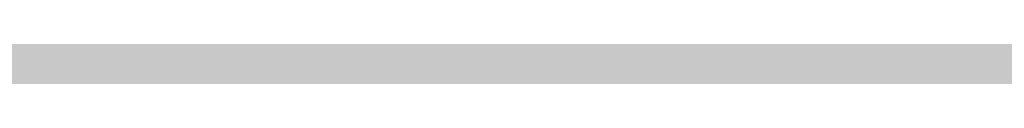
# Model space of a CAD drawing. Units: millimetres. Extents: x -22994 to 29398, y -19990 to 20176.
# Tile 89 of 135: x 229.428 to 230.597, y 83.505 to 83.535. Entities that reach past the tile are written whole.
import ezdxf
from ezdxf import colors
from ezdxf.entities.mleader import LeaderData, LeaderLine
from ezdxf.math import Vec2, Vec3

# ---------------------------------------------------------------- set-up
doc = ezdxf.new("R2010")
doc.units = ezdxf.units.MM
doc.header["$MEASUREMENT"] = 0
doc.layers.add('M-ANNO-TEXT', color=7, linetype='Continuous', lineweight=25)
doc.layers.add('M-DIMS', color=2, linetype='Continuous', lineweight=18)
doc.styles.get("Standard").update_dxf_attribs({"font": 'arial.ttf'})
doc.dimstyles.get("Standard").update_dxf_attribs({"dimtxt": 0.18, "dimasz": 10000, "dimexe": 0.18, "dimexo": 0.0625, "dimgap": 0.09, "dimtad": 0, "dimtih": 1, "dimtoh": 1, "dimdec": 0, "dimzin": 0, "dimdsep": 46, "dimtxsty": 'Standard', "dimcen": 0.09, "dimadec": 0, "dimazin": 0, "dimtfac": 1, "dimtdec": 0, "dimtofl": 0, "dimtmove": 0, "dimatfit": 3, "dimfxl": 1, "dimtolj": 1, "dimtzin": 0, "dimlwd": 30, "dimarcsym": 0})

# ---------------------------------------------------------------- blocks, each defined once
blk = doc.blocks.new('*D2')
at = {"layer": 'Defpoints', "color": 0, "transparency": 16777216}
for p in [(6.6773, 10.2713), (290.852, 10.2713), (290.852, -5.0787)]:
    blk.add_point(p, dxfattribs=at)
at = {"layer": 'M-DIMS', "color": 0, "lineweight": -2, "transparency": 16777216}
for p, q in [((6.6773, 10.2088), (6.6773, -5.2587)), ((290.852, 10.2088), (290.852, -5.2587))]:
    blk.add_line(p, q, dxfattribs=at)
at = {"layer": 'M-DIMS', "color": 0, "lineweight": 30, "transparency": 16777216}
for p, q in [((-9993.3227, -5.0787), (-19993.3227, -5.0787)), ((10290.852, -5.0787), (20290.852, -5.0787))]:
    blk.add_line(p, q, dxfattribs=at)
at = {"layer": 'M-DIMS', "color": 0, "transparency": 16777216}
for points in [[(-9993.3227, 1661.5879), (-9993.3227, -1671.7454), (6.6773, -5.0787)], [(10290.852, 1661.5879), (10290.852, -1671.7454), (290.852, -5.0787)]]:
    blk.add_solid(points, dxfattribs=at)
at = {"layer": 'M-DIMS', "color": 0, "transparency": 16777216, "insert": (148.7647, -5.0787), "char_height": 0.18, "attachment_point": 5}
blk.add_mtext('\\A1;284.2', dxfattribs=at)
blk = doc.blocks.new('*D3')
at = {"layer": 'Defpoints', "color": 0, "transparency": 16777216}
for p in [(110.2647, 204.1654), (110.2647, 176.3662), (95.8327, 127.967)]:
    blk.add_point(p, dxfattribs=at)
at = {"layer": 'M-DIMS', "color": 0, "lineweight": -2, "transparency": 16777216}
for p, q in [((95.8327, 128.0295), (95.8327, 204.3454)), ((110.2647, 176.4287), (110.2647, 204.3454))]:
    blk.add_line(p, q, dxfattribs=at)
at = {"layer": 'M-DIMS', "color": 0, "lineweight": 30, "transparency": 16777216}
for p, q in [((-9904.1673, 204.1654), (-19904.1673, 204.1654)), ((10110.2647, 204.1654), (20110.2647, 204.1654))]:
    blk.add_line(p, q, dxfattribs=at)
at = {"layer": 'M-DIMS', "color": 0, "transparency": 16777216}
for points in [[(-9904.1673, 1870.8321), (-9904.1673, -1462.5013), (95.8327, 204.1654)], [(10110.2647, 1870.8321), (10110.2647, -1462.5013), (110.2647, 204.1654)]]:
    blk.add_solid(points, dxfattribs=at)
at = {"layer": 'M-DIMS', "color": 0, "transparency": 16777216, "insert": (103.0487, 204.1654), "char_height": 0.18, "attachment_point": 5}
blk.add_mtext('\\A1;14.432', dxfattribs=at)
blk = doc.blocks.new('*D4')
at = {"layer": 'Defpoints', "color": 0, "transparency": 16777216}
for p in [(116.2647, 204.1654), (110.2647, 176.3662), (116.2647, 176.3662)]:
    blk.add_point(p, dxfattribs=at)
at = {"layer": 'M-DIMS', "color": 0, "lineweight": -2, "transparency": 16777216}
for p, q in [((110.2647, 176.4287), (110.2647, 204.3454)), ((116.2647, 176.4287), (116.2647, 204.3454))]:
    blk.add_line(p, q, dxfattribs=at)
at = {"layer": 'M-DIMS', "color": 0, "lineweight": 30, "transparency": 16777216}
for p, q in [((-9889.7353, 204.1654), (-19889.7353, 204.1654)), ((10116.2647, 204.1654), (20116.2647, 204.1654))]:
    blk.add_line(p, q, dxfattribs=at)
at = {"layer": 'M-DIMS', "color": 0, "transparency": 16777216}
for points in [[(-9889.7353, 1870.8321), (-9889.7353, -1462.5013), (110.2647, 204.1654)], [(10116.2647, 1870.8321), (10116.2647, -1462.5013), (116.2647, 204.1654)]]:
    blk.add_solid(points, dxfattribs=at)
at = {"layer": 'M-DIMS', "color": 0, "transparency": 16777216, "insert": (113.2647, 204.1654), "char_height": 0.18, "attachment_point": 5}
blk.add_mtext('\\A1;6', dxfattribs=at)
blk = doc.blocks.new('*D5')
at = {"layer": 'Defpoints', "color": 0, "transparency": 16777216}
for p in [(181.2647, 204.1654), (116.2647, 176.3662), (181.2647, 176.3662)]:
    blk.add_point(p, dxfattribs=at)
at = {"layer": 'M-DIMS', "color": 0, "lineweight": -2, "transparency": 16777216}
for p, q in [((116.2647, 176.4287), (116.2647, 204.3454)), ((181.2647, 176.4287), (181.2647, 204.3454))]:
    blk.add_line(p, q, dxfattribs=at)
at = {"layer": 'M-DIMS', "color": 0, "lineweight": 30, "transparency": 16777216}
for p, q in [((-9883.7353, 204.1654), (-19883.7353, 204.1654)), ((10181.2647, 204.1654), (20181.2647, 204.1654))]:
    blk.add_line(p, q, dxfattribs=at)
at = {"layer": 'M-DIMS', "color": 0, "transparency": 16777216}
for points in [[(-9883.7353, 1870.8321), (-9883.7353, -1462.5013), (116.2647, 204.1654)], [(10181.2647, 1870.8321), (10181.2647, -1462.5013), (181.2647, 204.1654)]]:
    blk.add_solid(points, dxfattribs=at)
at = {"layer": 'M-DIMS', "color": 0, "transparency": 16777216, "insert": (148.7647, 204.1654), "char_height": 0.18, "attachment_point": 5}
blk.add_mtext('\\A1;65', dxfattribs=at)
blk = doc.blocks.new('*D6')
at = {"layer": 'Defpoints', "color": 0, "transparency": 16777216}
for p in [(187.2647, 204.1654), (181.2647, 176.3662), (187.2647, 176.3662)]:
    blk.add_point(p, dxfattribs=at)
at = {"layer": 'M-DIMS', "color": 0, "lineweight": -2, "transparency": 16777216}
for p, q in [((181.2647, 176.4287), (181.2647, 204.3454)), ((187.2647, 176.4287), (187.2647, 204.3454))]:
    blk.add_line(p, q, dxfattribs=at)
at = {"layer": 'M-DIMS', "color": 0, "lineweight": 30, "transparency": 16777216}
for p, q in [((-9818.7353, 204.1654), (-19818.7353, 204.1654)), ((10187.2647, 204.1654), (20187.2647, 204.1654))]:
    blk.add_line(p, q, dxfattribs=at)
at = {"layer": 'M-DIMS', "color": 0, "transparency": 16777216}
for points in [[(-9818.7353, 1870.8321), (-9818.7353, -1462.5013), (181.2647, 204.1654)], [(10187.2647, 1870.8321), (10187.2647, -1462.5013), (187.2647, 204.1654)]]:
    blk.add_solid(points, dxfattribs=at)
at = {"layer": 'M-DIMS', "color": 0, "transparency": 16777216, "insert": (184.2647, 204.1654), "char_height": 0.18, "attachment_point": 5}
blk.add_mtext('\\A1;6', dxfattribs=at)
blk = doc.blocks.new('*D7')
at = {"layer": 'Defpoints', "color": 0, "transparency": 16777216}
for p in [(201.6967, 204.1654), (187.2647, 176.3662), (201.6967, 127.967)]:
    blk.add_point(p, dxfattribs=at)
at = {"layer": 'M-DIMS', "color": 0, "lineweight": -2, "transparency": 16777216}
for p, q in [((187.2647, 176.4287), (187.2647, 204.3454)), ((201.6967, 128.0295), (201.6967, 204.3454))]:
    blk.add_line(p, q, dxfattribs=at)
at = {"layer": 'M-DIMS', "color": 0, "lineweight": 30, "transparency": 16777216}
for p, q in [((-9812.7353, 204.1654), (-19812.7353, 204.1654)), ((10201.6967, 204.1654), (20201.6967, 204.1654))]:
    blk.add_line(p, q, dxfattribs=at)
at = {"layer": 'M-DIMS', "color": 0, "transparency": 16777216}
for points in [[(-9812.7353, 1870.8321), (-9812.7353, -1462.5013), (187.2647, 204.1654)], [(10201.6967, 1870.8321), (10201.6967, -1462.5013), (201.6967, 204.1654)]]:
    blk.add_solid(points, dxfattribs=at)
at = {"layer": 'M-DIMS', "color": 0, "transparency": 16777216, "insert": (194.4807, 204.1654), "char_height": 0.18, "attachment_point": 5}
blk.add_mtext('\\A1;14.432', dxfattribs=at)
blk = doc.blocks.new('*D8')
at = {"layer": 'Defpoints', "color": 0, "transparency": 16777216}
for p in [(227.6485, 204.1654), (227.6485, 146.7296), (201.6967, 127.967)]:
    blk.add_point(p, dxfattribs=at)
at = {"layer": 'M-DIMS', "color": 0, "lineweight": -2, "transparency": 16777216}
for p, q in [((201.6967, 128.0295), (201.6967, 204.3454)), ((227.6485, 146.7921), (227.6485, 204.3454))]:
    blk.add_line(p, q, dxfattribs=at)
at = {"layer": 'M-DIMS', "color": 0, "lineweight": 30, "transparency": 16777216}
for p, q in [((-9798.3033, 204.1654), (-19798.3033, 204.1654)), ((10227.6485, 204.1654), (20227.6485, 204.1654))]:
    blk.add_line(p, q, dxfattribs=at)
at = {"layer": 'M-DIMS', "color": 0, "transparency": 16777216}
for points in [[(-9798.3033, 1870.8321), (-9798.3033, -1462.5013), (201.6967, 204.1654)], [(10227.6485, 1870.8321), (10227.6485, -1462.5013), (227.6485, 204.1654)]]:
    blk.add_solid(points, dxfattribs=at)
at = {"layer": 'M-DIMS', "color": 0, "transparency": 16777216, "insert": (214.6726, 204.1654), "char_height": 0.18, "attachment_point": 5}
blk.add_mtext('\\A1;25.95', dxfattribs=at)
blk = doc.blocks.new('*D9')
at = {"layer": 'Defpoints', "color": 0, "transparency": 16777216}
for p in [(187.2647, 176.3662), (306.202, 176.3662), (290.852, 10.2713)]:
    blk.add_point(p, dxfattribs=at)
at = {"layer": 'M-DIMS', "color": 0, "lineweight": 30, "transparency": 16777216}
for p, q in [((306.202, 10176.3662), (306.202, 20176.3662)), ((306.202, -9989.7287), (306.202, -19989.7287))]:
    blk.add_line(p, q, dxfattribs=at)
at = {"layer": 'M-DIMS', "color": 0, "lineweight": -2, "transparency": 16777216}
for p, q in [((187.3272, 176.3662), (306.382, 176.3662)), ((290.9145, 10.2713), (306.382, 10.2713))]:
    blk.add_line(p, q, dxfattribs=at)
at = {"layer": 'M-DIMS', "color": 0, "transparency": 16777216}
for points in [[(-1360.4646, 10176.3662), (1972.8687, 10176.3662), (306.202, 176.3662)], [(-1360.4646, -9989.7287), (1972.8687, -9989.7287), (306.202, 10.2713)]]:
    blk.add_solid(points, dxfattribs=at)
at = {"layer": 'M-DIMS', "color": 0, "transparency": 16777216, "insert": (306.202, 93.3187), "char_height": 0.18, "attachment_point": 5}
blk.add_mtext('\\A1;166.1', dxfattribs=at)
blk = doc.blocks.new('*D10')
at = {"layer": 'Defpoints', "color": 0, "transparency": 16777216}
for p in [(125.6498, 136.0713), (133.3459, 136.0713), (133.3459, -5.0787)]:
    blk.add_point(p, dxfattribs=at)
at = {"layer": 'M-DIMS', "color": 0, "lineweight": -2, "transparency": 16777216}
for p, q in [((125.6498, 136.0088), (125.6498, -5.2587)), ((133.3459, 136.0088), (133.3459, -5.2587))]:
    blk.add_line(p, q, dxfattribs=at)
at = {"layer": 'M-DIMS', "color": 0, "lineweight": 30, "transparency": 16777216}
for p, q in [((-9874.3502, -5.0787), (-19874.3502, -5.0787)), ((10133.3459, -5.0787), (20133.3459, -5.0787))]:
    blk.add_line(p, q, dxfattribs=at)
at = {"layer": 'M-DIMS', "color": 0, "transparency": 16777216}
for points in [[(-9874.3502, 1661.5879), (-9874.3502, -1671.7454), (125.6498, -5.0787)], [(10133.3459, 1661.5879), (10133.3459, -1671.7454), (133.3459, -5.0787)]]:
    blk.add_solid(points, dxfattribs=at)
at = {"layer": 'M-DIMS', "color": 0, "transparency": 16777216, "insert": (129.4978, -5.0787), "char_height": 0.18, "attachment_point": 5}
blk.add_mtext('\\A1;7.696', dxfattribs=at)
blk = doc.blocks.new('*D11')
at = {"layer": 'Defpoints', "color": 0, "transparency": 16777216}
for p in [(133.3459, 136.0713), (135.6498, 136.0713), (135.6498, -5.0787)]:
    blk.add_point(p, dxfattribs=at)
at = {"layer": 'M-DIMS', "color": 0, "lineweight": -2, "transparency": 16777216}
for p, q in [((133.3459, 136.0088), (133.3459, -5.2587)), ((135.6498, 136.0088), (135.6498, -5.2587))]:
    blk.add_line(p, q, dxfattribs=at)
at = {"layer": 'M-DIMS', "color": 0, "lineweight": 30, "transparency": 16777216}
for p, q in [((-9866.6541, -5.0787), (-19866.6541, -5.0787)), ((10135.6498, -5.0787), (20135.6498, -5.0787))]:
    blk.add_line(p, q, dxfattribs=at)
at = {"layer": 'M-DIMS', "color": 0, "transparency": 16777216}
for points in [[(-9866.6541, 1661.5879), (-9866.6541, -1671.7454), (133.3459, -5.0787)], [(10135.6498, 1661.5879), (10135.6498, -1671.7454), (135.6498, -5.0787)]]:
    blk.add_solid(points, dxfattribs=at)
at = {"layer": 'M-DIMS', "color": 0, "transparency": 16777216, "insert": (134.4978, -5.0787), "char_height": 0.18, "attachment_point": 5}
blk.add_mtext('\\A1;2.304', dxfattribs=at)
blk = doc.blocks.new('*D12')
at = {"layer": 'Defpoints', "color": 0, "transparency": 16777216}
for p in [(135.6498, 136.0713), (145.6498, 136.0713), (145.6498, -5.0787)]:
    blk.add_point(p, dxfattribs=at)
at = {"layer": 'M-DIMS', "color": 0, "lineweight": -2, "transparency": 16777216}
for p, q in [((135.6498, 136.0088), (135.6498, -5.2587)), ((145.6498, 136.0088), (145.6498, -5.2587))]:
    blk.add_line(p, q, dxfattribs=at)
at = {"layer": 'M-DIMS', "color": 0, "lineweight": 30, "transparency": 16777216}
for p, q in [((-9864.3502, -5.0787), (-19864.3502, -5.0787)), ((10145.6498, -5.0787), (20145.6498, -5.0787))]:
    blk.add_line(p, q, dxfattribs=at)
at = {"layer": 'M-DIMS', "color": 0, "transparency": 16777216}
for points in [[(-9864.3502, 1661.5879), (-9864.3502, -1671.7454), (135.6498, -5.0787)], [(10145.6498, 1661.5879), (10145.6498, -1671.7454), (145.6498, -5.0787)]]:
    blk.add_solid(points, dxfattribs=at)
at = {"layer": 'M-DIMS', "color": 0, "transparency": 16777216, "insert": (140.6498, -5.0787), "char_height": 0.18, "attachment_point": 5}
blk.add_mtext('\\A1;10', dxfattribs=at)
blk = doc.blocks.new('*D13')
at = {"layer": 'Defpoints', "color": 0, "transparency": 16777216}
for p in [(145.6498, 136.0713), (155.6498, 136.0713), (155.6498, -5.0787)]:
    blk.add_point(p, dxfattribs=at)
at = {"layer": 'M-DIMS', "color": 0, "lineweight": -2, "transparency": 16777216}
for p, q in [((145.6498, 136.0088), (145.6498, -5.2587)), ((155.6498, 136.0088), (155.6498, -5.2587))]:
    blk.add_line(p, q, dxfattribs=at)
at = {"layer": 'M-DIMS', "color": 0, "lineweight": 30, "transparency": 16777216}
for p, q in [((-9854.3502, -5.0787), (-19854.3502, -5.0787)), ((10155.6498, -5.0787), (20155.6498, -5.0787))]:
    blk.add_line(p, q, dxfattribs=at)
at = {"layer": 'M-DIMS', "color": 0, "transparency": 16777216}
for points in [[(-9854.3502, 1661.5879), (-9854.3502, -1671.7454), (145.6498, -5.0787)], [(10155.6498, 1661.5879), (10155.6498, -1671.7454), (155.6498, -5.0787)]]:
    blk.add_solid(points, dxfattribs=at)
at = {"layer": 'M-DIMS', "color": 0, "transparency": 16777216, "insert": (150.6498, -5.0787), "char_height": 0.18, "attachment_point": 5}
blk.add_mtext('\\A1;10', dxfattribs=at)
blk = doc.blocks.new('*D14')
at = {"layer": 'Defpoints', "color": 0, "transparency": 16777216}
for p in [(155.6498, 136.0713), (165.6498, 136.0713), (165.6498, -5.0787)]:
    blk.add_point(p, dxfattribs=at)
at = {"layer": 'M-DIMS', "color": 0, "lineweight": -2, "transparency": 16777216}
for p, q in [((155.6498, 136.0088), (155.6498, -5.2587)), ((165.6498, 136.0088), (165.6498, -5.2587))]:
    blk.add_line(p, q, dxfattribs=at)
at = {"layer": 'M-DIMS', "color": 0, "lineweight": 30, "transparency": 16777216}
for p, q in [((-9844.3502, -5.0787), (-19844.3502, -5.0787)), ((10165.6498, -5.0787), (20165.6498, -5.0787))]:
    blk.add_line(p, q, dxfattribs=at)
at = {"layer": 'M-DIMS', "color": 0, "transparency": 16777216}
for points in [[(-9844.3502, 1661.5879), (-9844.3502, -1671.7454), (155.6498, -5.0787)], [(10165.6498, 1661.5879), (10165.6498, -1671.7454), (165.6498, -5.0787)]]:
    blk.add_solid(points, dxfattribs=at)
at = {"layer": 'M-DIMS', "color": 0, "transparency": 16777216, "insert": (160.6498, -5.0787), "char_height": 0.18, "attachment_point": 5}
blk.add_mtext('\\A1;10', dxfattribs=at)
blk = doc.blocks.new('*D15')
at = {"layer": 'Defpoints', "color": 0, "transparency": 16777216}
for p in [(173.3459, 154.788), (173.3459, 136.0713), (306.202, 136.0713)]:
    blk.add_point(p, dxfattribs=at)
at = {"layer": 'M-DIMS', "color": 0, "lineweight": 30, "transparency": 16777216}
for p, q in [((306.202, 10154.788), (306.202, 20154.788)), ((306.202, -9863.9287), (306.202, -19863.9287))]:
    blk.add_line(p, q, dxfattribs=at)
at = {"layer": 'M-DIMS', "color": 0, "lineweight": -2, "transparency": 16777216}
for p, q in [((173.4084, 154.788), (306.382, 154.788)), ((173.4084, 136.0713), (306.382, 136.0713))]:
    blk.add_line(p, q, dxfattribs=at)
at = {"layer": 'M-DIMS', "color": 0, "transparency": 16777216}
for points in [[(-1360.4646, 10154.788), (1972.8687, 10154.788), (306.202, 154.788)], [(-1360.4646, -9863.9287), (1972.8687, -9863.9287), (306.202, 136.0713)]]:
    blk.add_solid(points, dxfattribs=at)
at = {"layer": 'M-DIMS', "color": 0, "transparency": 16777216, "insert": (306.202, 145.4297), "char_height": 0.18, "attachment_point": 5}
blk.add_mtext('\\A1;18.717', dxfattribs=at)
blk = doc.blocks.new('*D16')
at = {"layer": 'Defpoints', "color": 0, "transparency": 16777216}
for p in [(120.1702, 204.1654), (110.4658, 48.0349), (120.1702, 48.0349)]:
    blk.add_point(p, dxfattribs=at)
at = {"layer": 'M-DIMS', "color": 0, "lineweight": -2, "transparency": 16777216}
for p, q in [((110.4658, 48.0974), (110.4658, 204.3454)), ((120.1702, 48.0974), (120.1702, 204.3454))]:
    blk.add_line(p, q, dxfattribs=at)
at = {"layer": 'M-DIMS', "color": 0, "lineweight": 30, "transparency": 16777216}
for p, q in [((-9889.5342, 204.1654), (-19889.5342, 204.1654)), ((10120.1702, 204.1654), (20120.1702, 204.1654))]:
    blk.add_line(p, q, dxfattribs=at)
at = {"layer": 'M-DIMS', "color": 0, "transparency": 16777216}
for points in [[(-9889.5342, 1870.8321), (-9889.5342, -1462.5013), (110.4658, 204.1654)], [(10120.1702, 1870.8321), (10120.1702, -1462.5013), (120.1702, 204.1654)]]:
    blk.add_solid(points, dxfattribs=at)
at = {"layer": 'M-DIMS', "color": 0, "transparency": 16777216, "insert": (115.318, 204.1654), "char_height": 0.18, "attachment_point": 5}
blk.add_mtext('\\A1;9.704', dxfattribs=at)
blk = doc.blocks.new('*D17')
at = {"layer": 'Defpoints', "color": 0, "transparency": 16777216}
for p in [(126.1702, 204.1654), (120.1702, 48.0349), (126.1702, 48.0349)]:
    blk.add_point(p, dxfattribs=at)
at = {"layer": 'M-DIMS', "color": 0, "lineweight": -2, "transparency": 16777216}
for p, q in [((120.1702, 48.0974), (120.1702, 204.3454)), ((126.1702, 48.0974), (126.1702, 204.3454))]:
    blk.add_line(p, q, dxfattribs=at)
at = {"layer": 'M-DIMS', "color": 0, "lineweight": 30, "transparency": 16777216}
for p, q in [((-9879.8298, 204.1654), (-19879.8298, 204.1654)), ((10126.1702, 204.1654), (20126.1702, 204.1654))]:
    blk.add_line(p, q, dxfattribs=at)
at = {"layer": 'M-DIMS', "color": 0, "transparency": 16777216}
for points in [[(-9879.8298, 1870.8321), (-9879.8298, -1462.5013), (120.1702, 204.1654)], [(10126.1702, 1870.8321), (10126.1702, -1462.5013), (126.1702, 204.1654)]]:
    blk.add_solid(points, dxfattribs=at)
at = {"layer": 'M-DIMS', "color": 0, "transparency": 16777216, "insert": (123.1702, 204.1654), "char_height": 0.18, "attachment_point": 5}
blk.add_mtext('\\A1;6', dxfattribs=at)
blk = doc.blocks.new('*D18')
at = {"layer": 'Defpoints', "color": 0, "transparency": 16777216}
for p in [(132.1702, 204.1654), (126.1702, 48.0349), (132.1702, 48.0349)]:
    blk.add_point(p, dxfattribs=at)
at = {"layer": 'M-DIMS', "color": 0, "lineweight": -2, "transparency": 16777216}
for p, q in [((126.1702, 48.0974), (126.1702, 204.3454)), ((132.1702, 48.0974), (132.1702, 204.3454))]:
    blk.add_line(p, q, dxfattribs=at)
at = {"layer": 'M-DIMS', "color": 0, "lineweight": 30, "transparency": 16777216}
for p, q in [((-9873.8298, 204.1654), (-19873.8298, 204.1654)), ((10132.1702, 204.1654), (20132.1702, 204.1654))]:
    blk.add_line(p, q, dxfattribs=at)
at = {"layer": 'M-DIMS', "color": 0, "transparency": 16777216}
for points in [[(-9873.8298, 1870.8321), (-9873.8298, -1462.5013), (126.1702, 204.1654)], [(10132.1702, 1870.8321), (10132.1702, -1462.5013), (132.1702, 204.1654)]]:
    blk.add_solid(points, dxfattribs=at)
at = {"layer": 'M-DIMS', "color": 0, "transparency": 16777216, "insert": (129.1702, 204.1654), "char_height": 0.18, "attachment_point": 5}
blk.add_mtext('\\A1;6', dxfattribs=at)
blk = doc.blocks.new('*D19')
at = {"layer": 'Defpoints', "color": 0, "transparency": 16777216}
for p in [(138.1702, 204.1654), (132.1702, 48.0349), (138.1702, 48.0349)]:
    blk.add_point(p, dxfattribs=at)
at = {"layer": 'M-DIMS', "color": 0, "lineweight": -2, "transparency": 16777216}
for p, q in [((132.1702, 48.0974), (132.1702, 204.3454)), ((138.1702, 48.0974), (138.1702, 204.3454))]:
    blk.add_line(p, q, dxfattribs=at)
at = {"layer": 'M-DIMS', "color": 0, "lineweight": 30, "transparency": 16777216}
for p, q in [((-9867.8298, 204.1654), (-19867.8298, 204.1654)), ((10138.1702, 204.1654), (20138.1702, 204.1654))]:
    blk.add_line(p, q, dxfattribs=at)
at = {"layer": 'M-DIMS', "color": 0, "transparency": 16777216}
for points in [[(-9867.8298, 1870.8321), (-9867.8298, -1462.5013), (132.1702, 204.1654)], [(10138.1702, 1870.8321), (10138.1702, -1462.5013), (138.1702, 204.1654)]]:
    blk.add_solid(points, dxfattribs=at)
at = {"layer": 'M-DIMS', "color": 0, "transparency": 16777216, "insert": (135.1702, 204.1654), "char_height": 0.18, "attachment_point": 5}
blk.add_mtext('\\A1;6', dxfattribs=at)
blk = doc.blocks.new('*D20')
at = {"layer": 'Defpoints', "color": 0, "transparency": 16777216}
for p in [(144.1702, 204.1654), (138.1702, 48.0349), (144.1702, 48.0349)]:
    blk.add_point(p, dxfattribs=at)
at = {"layer": 'M-DIMS', "color": 0, "lineweight": -2, "transparency": 16777216}
for p, q in [((138.1702, 48.0974), (138.1702, 204.3454)), ((144.1702, 48.0974), (144.1702, 204.3454))]:
    blk.add_line(p, q, dxfattribs=at)
at = {"layer": 'M-DIMS', "color": 0, "lineweight": 30, "transparency": 16777216}
for p, q in [((-9861.8298, 204.1654), (-19861.8298, 204.1654)), ((10144.1702, 204.1654), (20144.1702, 204.1654))]:
    blk.add_line(p, q, dxfattribs=at)
at = {"layer": 'M-DIMS', "color": 0, "transparency": 16777216}
for points in [[(-9861.8298, 1870.8321), (-9861.8298, -1462.5013), (138.1702, 204.1654)], [(10144.1702, 1870.8321), (10144.1702, -1462.5013), (144.1702, 204.1654)]]:
    blk.add_solid(points, dxfattribs=at)
at = {"layer": 'M-DIMS', "color": 0, "transparency": 16777216, "insert": (141.1702, 204.1654), "char_height": 0.18, "attachment_point": 5}
blk.add_mtext('\\A1;6', dxfattribs=at)
blk = doc.blocks.new('*D21')
at = {"layer": 'Defpoints', "color": 0, "transparency": 16777216}
for p in [(149.1157, 204.1654), (144.1702, 48.0349), (149.1157, 48.0349)]:
    blk.add_point(p, dxfattribs=at)
at = {"layer": 'M-DIMS', "color": 0, "lineweight": -2, "transparency": 16777216}
for p, q in [((144.1702, 48.0974), (144.1702, 204.3454)), ((149.1157, 48.0974), (149.1157, 204.3454))]:
    blk.add_line(p, q, dxfattribs=at)
at = {"layer": 'M-DIMS', "color": 0, "lineweight": 30, "transparency": 16777216}
for p, q in [((-9855.8298, 204.1654), (-19855.8298, 204.1654)), ((10149.1157, 204.1654), (20149.1157, 204.1654))]:
    blk.add_line(p, q, dxfattribs=at)
at = {"layer": 'M-DIMS', "color": 0, "transparency": 16777216}
for points in [[(-9855.8298, 1870.8321), (-9855.8298, -1462.5013), (144.1702, 204.1654)], [(10149.1157, 1870.8321), (10149.1157, -1462.5013), (149.1157, 204.1654)]]:
    blk.add_solid(points, dxfattribs=at)
at = {"layer": 'M-DIMS', "color": 0, "transparency": 16777216, "insert": (146.6429, 204.1654), "char_height": 0.18, "attachment_point": 5}
blk.add_mtext('\\A1;4.945', dxfattribs=at)
blk = doc.blocks.new('*D22')
at = {"layer": 'Defpoints', "color": 0, "transparency": 16777216}
for p in [(149.1157, 30.9895), (155.1157, 30.9895), (155.1157, -5.0787)]:
    blk.add_point(p, dxfattribs=at)
at = {"layer": 'M-DIMS', "color": 0, "lineweight": -2, "transparency": 16777216}
for p, q in [((149.1157, 30.927), (149.1157, -5.2587)), ((155.1157, 30.927), (155.1157, -5.2587))]:
    blk.add_line(p, q, dxfattribs=at)
at = {"layer": 'M-DIMS', "color": 0, "lineweight": 30, "transparency": 16777216}
for p, q in [((-9850.8843, -5.0787), (-19850.8843, -5.0787)), ((10155.1157, -5.0787), (20155.1157, -5.0787))]:
    blk.add_line(p, q, dxfattribs=at)
at = {"layer": 'M-DIMS', "color": 0, "transparency": 16777216}
for points in [[(-9850.8843, 1661.5879), (-9850.8843, -1671.7454), (149.1157, -5.0787)], [(10155.1157, 1661.5879), (10155.1157, -1671.7454), (155.1157, -5.0787)]]:
    blk.add_solid(points, dxfattribs=at)
at = {"layer": 'M-DIMS', "color": 0, "transparency": 16777216, "insert": (152.1157, -5.0787), "char_height": 0.18, "attachment_point": 5}
blk.add_mtext('\\A1;6', dxfattribs=at)
blk = doc.blocks.new('*D23')
at = {"layer": 'Defpoints', "color": 0, "transparency": 16777216}
for p in [(155.1157, 30.9895), (161.1157, 30.9895), (161.1157, -5.0787)]:
    blk.add_point(p, dxfattribs=at)
at = {"layer": 'M-DIMS', "color": 0, "lineweight": -2, "transparency": 16777216}
for p, q in [((155.1157, 30.927), (155.1157, -5.2587)), ((161.1157, 30.927), (161.1157, -5.2587))]:
    blk.add_line(p, q, dxfattribs=at)
at = {"layer": 'M-DIMS', "color": 0, "lineweight": 30, "transparency": 16777216}
for p, q in [((-9844.8843, -5.0787), (-19844.8843, -5.0787)), ((10161.1157, -5.0787), (20161.1157, -5.0787))]:
    blk.add_line(p, q, dxfattribs=at)
at = {"layer": 'M-DIMS', "color": 0, "transparency": 16777216}
for points in [[(-9844.8843, 1661.5879), (-9844.8843, -1671.7454), (155.1157, -5.0787)], [(10161.1157, 1661.5879), (10161.1157, -1671.7454), (161.1157, -5.0787)]]:
    blk.add_solid(points, dxfattribs=at)
at = {"layer": 'M-DIMS', "color": 0, "transparency": 16777216, "insert": (158.1157, -5.0787), "char_height": 0.18, "attachment_point": 5}
blk.add_mtext('\\A1;6', dxfattribs=at)
blk = doc.blocks.new('*D24')
at = {"layer": 'Defpoints', "color": 0, "transparency": 16777216}
for p in [(161.1157, 30.9895), (166.4387, 30.9895), (166.4387, -5.0787)]:
    blk.add_point(p, dxfattribs=at)
at = {"layer": 'M-DIMS', "color": 0, "lineweight": -2, "transparency": 16777216}
for p, q in [((161.1157, 30.927), (161.1157, -5.2587)), ((166.4387, 30.927), (166.4387, -5.2587))]:
    blk.add_line(p, q, dxfattribs=at)
at = {"layer": 'M-DIMS', "color": 0, "lineweight": 30, "transparency": 16777216}
for p, q in [((-9838.8843, -5.0787), (-19838.8843, -5.0787)), ((10166.4387, -5.0787), (20166.4387, -5.0787))]:
    blk.add_line(p, q, dxfattribs=at)
at = {"layer": 'M-DIMS', "color": 0, "transparency": 16777216}
for points in [[(-9838.8843, 1661.5879), (-9838.8843, -1671.7454), (161.1157, -5.0787)], [(10166.4387, 1661.5879), (10166.4387, -1671.7454), (166.4387, -5.0787)]]:
    blk.add_solid(points, dxfattribs=at)
at = {"layer": 'M-DIMS', "color": 0, "transparency": 16777216, "insert": (163.7772, -5.0787), "char_height": 0.18, "attachment_point": 5}
blk.add_mtext('\\A1;5.323', dxfattribs=at)
blk = doc.blocks.new('*D25')
at = {"layer": 'Defpoints', "color": 0, "transparency": 16777216}
for p in [(166.4387, 30.9895), (172.4387, 30.9895), (172.4387, -5.0787)]:
    blk.add_point(p, dxfattribs=at)
at = {"layer": 'M-DIMS', "color": 0, "lineweight": -2, "transparency": 16777216}
for p, q in [((166.4387, 30.927), (166.4387, -5.2587)), ((172.4387, 30.927), (172.4387, -5.2587))]:
    blk.add_line(p, q, dxfattribs=at)
at = {"layer": 'M-DIMS', "color": 0, "lineweight": 30, "transparency": 16777216}
for p, q in [((-9833.5613, -5.0787), (-19833.5613, -5.0787)), ((10172.4387, -5.0787), (20172.4387, -5.0787))]:
    blk.add_line(p, q, dxfattribs=at)
at = {"layer": 'M-DIMS', "color": 0, "transparency": 16777216}
for points in [[(-9833.5613, 1661.5879), (-9833.5613, -1671.7454), (166.4387, -5.0787)], [(10172.4387, 1661.5879), (10172.4387, -1671.7454), (172.4387, -5.0787)]]:
    blk.add_solid(points, dxfattribs=at)
at = {"layer": 'M-DIMS', "color": 0, "transparency": 16777216, "insert": (169.4387, -5.0787), "char_height": 0.18, "attachment_point": 5}
blk.add_mtext('\\A1;6', dxfattribs=at)
blk = doc.blocks.new('*D26')
at = {"layer": 'Defpoints', "color": 0, "transparency": 16777216}
for p in [(172.4387, 30.9895), (178.4387, 30.9895), (178.4387, -5.0787)]:
    blk.add_point(p, dxfattribs=at)
at = {"layer": 'M-DIMS', "color": 0, "lineweight": -2, "transparency": 16777216}
for p, q in [((172.4387, 30.927), (172.4387, -5.2587)), ((178.4387, 30.927), (178.4387, -5.2587))]:
    blk.add_line(p, q, dxfattribs=at)
at = {"layer": 'M-DIMS', "color": 0, "lineweight": 30, "transparency": 16777216}
for p, q in [((-9827.5613, -5.0787), (-19827.5613, -5.0787)), ((10178.4387, -5.0787), (20178.4387, -5.0787))]:
    blk.add_line(p, q, dxfattribs=at)
at = {"layer": 'M-DIMS', "color": 0, "transparency": 16777216}
for points in [[(-9827.5613, 1661.5879), (-9827.5613, -1671.7454), (172.4387, -5.0787)], [(10178.4387, 1661.5879), (10178.4387, -1671.7454), (178.4387, -5.0787)]]:
    blk.add_solid(points, dxfattribs=at)
at = {"layer": 'M-DIMS', "color": 0, "transparency": 16777216, "insert": (175.4387, -5.0787), "char_height": 0.18, "attachment_point": 5}
blk.add_mtext('\\A1;6', dxfattribs=at)
blk = doc.blocks.new('*D27')
at = {"layer": 'Defpoints', "color": 0, "transparency": 16777216}
for p in [(178.4387, 30.9895), (188.1175, 30.9895), (188.1175, -5.0787)]:
    blk.add_point(p, dxfattribs=at)
at = {"layer": 'M-DIMS', "color": 0, "lineweight": -2, "transparency": 16777216}
for p, q in [((178.4387, 30.927), (178.4387, -5.2587)), ((188.1175, 30.927), (188.1175, -5.2587))]:
    blk.add_line(p, q, dxfattribs=at)
at = {"layer": 'M-DIMS', "color": 0, "lineweight": 30, "transparency": 16777216}
for p, q in [((-9821.5613, -5.0787), (-19821.5613, -5.0787)), ((10188.1175, -5.0787), (20188.1175, -5.0787))]:
    blk.add_line(p, q, dxfattribs=at)
at = {"layer": 'M-DIMS', "color": 0, "transparency": 16777216}
for points in [[(-9821.5613, 1661.5879), (-9821.5613, -1671.7454), (178.4387, -5.0787)], [(10188.1175, 1661.5879), (10188.1175, -1671.7454), (188.1175, -5.0787)]]:
    blk.add_solid(points, dxfattribs=at)
at = {"layer": 'M-DIMS', "color": 0, "transparency": 16777216, "insert": (183.2781, -5.0787), "char_height": 0.18, "attachment_point": 5}
blk.add_mtext('\\A1;9.679', dxfattribs=at)
blk = doc.blocks.new('*D28')
at = {"layer": 'Defpoints', "color": 0, "transparency": 16777216}
for p in [(188.1175, 48.0349), (306.202, 48.0349), (188.1175, 30.9895)]:
    blk.add_point(p, dxfattribs=at)
at = {"layer": 'M-DIMS', "color": 0, "lineweight": 30, "transparency": 16777216}
for p, q in [((306.202, 10048.0349), (306.202, 20048.0349)), ((306.202, -9969.0105), (306.202, -19969.0105))]:
    blk.add_line(p, q, dxfattribs=at)
at = {"layer": 'M-DIMS', "color": 0, "lineweight": -2, "transparency": 16777216}
for p, q in [((188.18, 48.0349), (306.382, 48.0349)), ((188.18, 30.9895), (306.382, 30.9895))]:
    blk.add_line(p, q, dxfattribs=at)
at = {"layer": 'M-DIMS', "color": 0, "transparency": 16777216}
for points in [[(-1360.4646, 10048.0349), (1972.8687, 10048.0349), (306.202, 48.0349)], [(-1360.4646, -9969.0105), (1972.8687, -9969.0105), (306.202, 30.9895)]]:
    blk.add_solid(points, dxfattribs=at)
at = {"layer": 'M-DIMS', "color": 0, "transparency": 16777216, "insert": (306.202, 39.5122), "char_height": 0.18, "attachment_point": 5}
blk.add_mtext('\\A1;17.045', dxfattribs=at)
blk = doc.blocks.new('*D29')
at = {"layer": 'Defpoints', "color": 0, "transparency": 16777216}
for p in [(36.8006, 80.045), (64.0296, 80.045)]:
    blk.add_point(p, dxfattribs=at)
at = {"layer": 'M-DIMS', "color": 0, "lineweight": -2, "transparency": 16777216}
for p, q in [((50.4151, 79.955), (50.4151, 80.135)), ((50.3251, 80.045), (50.5051, 80.045))]:
    blk.add_line(p, q, dxfattribs=at)
at = {"layer": 'M-DIMS', "color": 0, "lineweight": 30, "transparency": 16777216}
blk.add_line((20064.0296, 80.0303), (10064.0296, 80.0377), dxfattribs=at)
at = {"layer": 'M-DIMS', "color": 0, "transparency": 16777216}
blk.add_solid([(10064.0309, 1746.7043), (10064.0284, -1586.629), (64.0296, 80.045)], dxfattribs=at)
at = {"layer": 'M-DIMS', "color": 0, "transparency": 16777216, "insert": (20064.5213, 80.0303), "char_height": 0.18, "attachment_point": 5}
blk.add_mtext('\\A1;∅27.23', dxfattribs=at)
blk = doc.blocks.new('*D30')
at = {"layer": 'Defpoints', "color": 0, "transparency": 16777216}
for p in [(216.3148, 146.7291), (238.9821, 146.73)]:
    blk.add_point(p, dxfattribs=at)
at = {"layer": 'M-DIMS', "color": 0, "lineweight": 30, "transparency": 16777216}
blk.add_line((20238.9821, 147.4959), (10238.9821, 147.1129), dxfattribs=at)
at = {"layer": 'M-DIMS', "color": 0, "lineweight": -2, "transparency": 16777216}
for p, q in [((227.6485, 146.6396), (227.6485, 146.8196)), ((227.5585, 146.7296), (227.7385, 146.7296))]:
    blk.add_line(p, q, dxfattribs=at)
at = {"layer": 'M-DIMS', "color": 0, "transparency": 16777216}
blk.add_solid([(10238.9183, 1813.7796), (10239.0459, -1519.5537), (238.9821, 146.73)], dxfattribs=at)
at = {"layer": 'M-DIMS', "color": 0, "transparency": 16777216, "insert": (20239.5436, 147.4959), "char_height": 0.18, "attachment_point": 5}
blk.add_mtext('\\A1;∅22.667', dxfattribs=at)
blk = doc.blocks.new('*D31')
at = {"layer": 'Defpoints', "color": 0, "transparency": 16777216}
for p in [(223.1641, 146.7291), (232.1328, 146.73)]:
    blk.add_point(p, dxfattribs=at)
at = {"layer": 'M-DIMS', "color": 0, "lineweight": 30, "transparency": 16777216}
blk.add_line((20232.1327, 148.6656), (10232.1328, 147.6978), dxfattribs=at)
at = {"layer": 'M-DIMS', "color": 0, "lineweight": -2, "transparency": 16777216}
for p, q in [((227.6485, 146.6396), (227.6485, 146.8196)), ((227.5585, 146.7296), (227.7385, 146.7296))]:
    blk.add_line(p, q, dxfattribs=at)
at = {"layer": 'M-DIMS', "color": 0, "transparency": 16777216}
blk.add_solid([(10231.9715, 1814.3645), (10232.2941, -1518.9688), (232.1328, 146.73)], dxfattribs=at)
at = {"layer": 'M-DIMS', "color": 0, "transparency": 16777216, "insert": (20232.6245, 148.6656), "char_height": 0.18, "attachment_point": 5}
blk.add_mtext('\\A1;∅8.969', dxfattribs=at)
blk = doc.blocks.new('*D33')
at = {"layer": 'Defpoints', "color": 0, "transparency": 16777216}
for p in [(229.5613, 154.3773), (232.9972, 153.3509)]:
    blk.add_point(p, dxfattribs=at)
at = {"layer": 'M-DIMS', "color": 0, "lineweight": -2, "transparency": 16777216}
for p, q in [((229.5613, 154.2873), (229.5613, 154.4673)), ((229.4713, 154.3773), (229.6513, 154.3773))]:
    blk.add_line(p, q, dxfattribs=at)
at = {"layer": 'M-DIMS', "color": 0, "lineweight": 30, "transparency": 16777216}
for p, q in [((19396.3388, -5570.8378), (9814.668, -2708.7434)), ((29396.3388, -5570.8378), (19396.3388, -5570.8378))]:
    blk.add_line(p, q, dxfattribs=at)
at = {"layer": 'M-DIMS', "color": 0, "transparency": 16777216}
blk.add_solid([(10291.6837, -1111.7983), (9337.6523, -4305.6886), (232.9972, 153.3509)], dxfattribs=at)
at = {"layer": 'M-DIMS', "color": 0, "transparency": 16777216, "insert": (29397.0125, -5570.8378), "char_height": 0.18, "attachment_point": 5}
blk.add_mtext('\\A1;6X R3.586', dxfattribs=at)
blk = doc.blocks.new('*D36')
at = {"layer": 'Defpoints', "color": 0, "transparency": 16777216}
for p in [(46.39, 31.3035), (46.3875, 26.5934)]:
    blk.add_point(p, dxfattribs=at)
at = {"layer": 'M-DIMS', "color": 0, "lineweight": 30, "transparency": 16777216}
for p, q in [((57.1499, 20031.3006), (51.77, 10031.302)), ((10057.1499, 20031.3006), (57.1499, 20031.3006))]:
    blk.add_line(p, q, dxfattribs=at)
at = {"layer": 'M-DIMS', "color": 0, "lineweight": -2, "transparency": 16777216}
for p, q in [((46.3887, 28.8585), (46.3887, 29.0385)), ((46.2987, 28.9485), (46.4787, 28.9485))]:
    blk.add_line(p, q, dxfattribs=at)
at = {"layer": 'M-DIMS', "color": 0, "transparency": 16777216}
blk.add_solid([(-1614.8965, 10032.1987), (1718.4364, 10030.4054), (46.39, 31.3035)], dxfattribs=at)
at = {"layer": 'M-DIMS', "color": 0, "transparency": 16777216, "insert": (10057.5542, 20031.3006), "char_height": 0.18, "attachment_point": 5}
blk.add_mtext('\\A1;∅4.71', dxfattribs=at)
blk = doc.blocks.new('*D37')
at = {"layer": 'Defpoints', "color": 0, "transparency": 16777216}
for p in [(54.8343, 118.6145), (59.4936, 118.614)]:
    blk.add_point(p, dxfattribs=at)
at = {"layer": 'M-DIMS', "color": 0, "lineweight": -2, "transparency": 16777216}
for p, q in [((57.1639, 118.5243), (57.1639, 118.7043)), ((57.0739, 118.6143), (57.2539, 118.6143))]:
    blk.add_line(p, q, dxfattribs=at)
at = {"layer": 'M-DIMS', "color": 0, "lineweight": 30, "transparency": 16777216}
blk.add_line((20059.4934, 116.2531), (10059.4935, 117.4336), dxfattribs=at)
at = {"layer": 'M-DIMS', "color": 0, "transparency": 16777216}
blk.add_solid([(10059.6902, 1784.1002), (10059.2968, -1549.2331), (59.4936, 118.614)], dxfattribs=at)
at = {"layer": 'M-DIMS', "color": 0, "transparency": 16777216, "insert": (20059.9852, 116.2531), "char_height": 0.18, "attachment_point": 5}
blk.add_mtext('\\A1;∅4.659', dxfattribs=at)

msp = doc.modelspace()

# ---------------------------------------------------------------- dimensions: what is measured, and where the dimension line sits
at = {"layer": 'M-DIMS'}
for base, p1, p2, override, picture, middle in [((306.202, 176.3662), (290.852, 10.2713), (187.2647, 176.3662), {"dimdec": 1, "dimlfac": 1, "dimrnd": 0, "dimzin": 0, "dimdsep": 46, "dimlunit": 2}, '*D9', (306.202, 93.3187)), ((306.202, 136.0713), (173.3459, 154.788), (173.3459, 136.0713), {"dimdec": 3, "dimlfac": 1, "dimrnd": 0, "dimzin": 0, "dimdsep": 46, "dimlunit": 2}, '*D15', (306.202, 145.4297)), ((306.202, 48.0349), (188.1175, 30.9895), (188.1175, 48.0349), {"dimdec": 3, "dimlfac": 1, "dimrnd": 0, "dimzin": 0, "dimdsep": 46, "dimlunit": 2}, '*D28', (306.202, 39.5122))]:
    dim = msp.add_linear_dim(base=base, p1=p1, p2=p2, angle=90, dimstyle='Standard', override=override, dxfattribs=at)
    dim.commit()
    dim.dimension.update_dxf_attribs({"geometry": picture, "text_midpoint": middle})
for p1, p2, override, picture, middle in [((46.3875, 26.5934), (46.39, 31.3035), {"dimdec": 2, "dimlfac": 1, "dimrnd": 0, "dimzin": 0, "dimdsep": 46, "dimlunit": 2}, '*D36', (10057.5542, 20031.3006)), ((223.1641, 146.7291), (232.1328, 146.73), {"dimdec": 3, "dimlfac": 1, "dimrnd": 0, "dimzin": 0, "dimdsep": 46, "dimlunit": 2}, '*D31', (20232.1327, 148.6656)), ((216.3148, 146.7291), (238.9821, 146.73), {"dimdec": 3, "dimlfac": 1, "dimrnd": 0, "dimzin": 0, "dimdsep": 46, "dimlunit": 2}, '*D30', (20238.9821, 147.4959))]:
    dim = msp.add_diameter_dim_2p(p1=p1, p2=p2, dimstyle='Standard', override=override, dxfattribs=at)
    dim.commit()
    dim.dimension.update_dxf_attribs({"geometry": picture, "text_midpoint": middle, "dimtype": 163})
for base, p1, p2, override, picture, middle in [((110.2647, 204.1654), (95.8327, 127.967), (110.2647, 176.3662), {"dimdec": 3, "dimlfac": 1, "dimrnd": 0, "dimzin": 0, "dimdsep": 46, "dimlunit": 2}, '*D3', (103.0487, 204.1654)), ((116.2647, 204.1654), (110.2647, 176.3662), (116.2647, 176.3662), {"dimdec": 0, "dimlfac": 1, "dimrnd": 0, "dimzin": 0, "dimdsep": 46, "dimlunit": 2}, '*D4', (113.2647, 204.1654)), ((120.1702, 204.1654), (110.4658, 48.0349), (120.1702, 48.0349), {"dimdec": 3, "dimlfac": 1, "dimrnd": 0, "dimzin": 0, "dimdsep": 46, "dimlunit": 2}, '*D16', (115.318, 204.1654)), ((181.2647, 204.1654), (116.2647, 176.3662), (181.2647, 176.3662), {"dimdec": 0, "dimlfac": 1, "dimrnd": 0, "dimzin": 0, "dimdsep": 46, "dimlunit": 2}, '*D5', (148.7647, 204.1654)), ((126.1702, 204.1654), (120.1702, 48.0349), (126.1702, 48.0349), {"dimdec": 0, "dimlfac": 1, "dimrnd": 0, "dimzin": 0, "dimdsep": 46, "dimlunit": 2}, '*D17', (123.1702, 204.1654)), ((132.1702, 204.1654), (126.1702, 48.0349), (132.1702, 48.0349), {"dimdec": 0, "dimlfac": 1, "dimrnd": 0, "dimzin": 0, "dimdsep": 46, "dimlunit": 2}, '*D18', (129.1702, 204.1654)), ((138.1702, 204.1654), (132.1702, 48.0349), (138.1702, 48.0349), {"dimdec": 0, "dimlfac": 1, "dimrnd": 0, "dimzin": 0, "dimdsep": 46, "dimlunit": 2}, '*D19', (135.1702, 204.1654)), ((144.1702, 204.1654), (138.1702, 48.0349), (144.1702, 48.0349), {"dimdec": 0, "dimlfac": 1, "dimrnd": 0, "dimzin": 0, "dimdsep": 46, "dimlunit": 2}, '*D20', (141.1702, 204.1654)), ((149.11567, 204.16539), (144.17023, 48.03494), (149.11567, 48.03494), {"dimdec": 3, "dimlfac": 1, "dimrnd": 0, "dimzin": 0, "dimdsep": 46, "dimlunit": 2}, '*D21', (146.64295, 204.16539)), ((187.2647, 204.1654), (181.2647, 176.3662), (187.2647, 176.3662), {"dimdec": 0, "dimlfac": 1, "dimrnd": 0, "dimzin": 0, "dimdsep": 46, "dimlunit": 2}, '*D6', (184.2647, 204.1654)), ((201.6967, 204.1654), (187.2647, 176.3662), (201.6967, 127.967), {"dimdec": 3, "dimlfac": 1, "dimrnd": 0, "dimzin": 0, "dimdsep": 46, "dimlunit": 2}, '*D7', (194.4807, 204.1654)), ((227.6485, 204.1654), (201.6967, 127.967), (227.6485, 146.7296), {"dimdec": 2, "dimlfac": 1, "dimrnd": 0, "dimzin": 0, "dimdsep": 46, "dimlunit": 2}, '*D8', (214.6726, 204.1654)), ((290.852, -5.0787), (6.6773, 10.2713), (290.852, 10.2713), {"dimdec": 1, "dimlfac": 1, "dimrnd": 0, "dimzin": 0, "dimdsep": 46, "dimlunit": 2}, '*D2', (148.7647, -5.0787)), ((133.3459, -5.0787), (125.6498, 136.0713), (133.3459, 136.0713), {"dimdec": 3, "dimlfac": 1, "dimrnd": 0, "dimzin": 0, "dimdsep": 46, "dimlunit": 2}, '*D10', (129.4978, -5.0787)), ((135.6498, -5.0787), (133.3459, 136.0713), (135.6498, 136.0713), {"dimdec": 3, "dimlfac": 1, "dimrnd": 0, "dimzin": 0, "dimdsep": 46, "dimlunit": 2}, '*D11', (134.4978, -5.0787)), ((145.6498, -5.0787), (135.6498, 136.0713), (145.6498, 136.0713), {"dimdec": 0, "dimlfac": 1, "dimrnd": 0, "dimzin": 0, "dimdsep": 46, "dimlunit": 2}, '*D12', (140.6498, -5.0787)), ((155.6498, -5.0787), (145.6498, 136.0713), (155.6498, 136.0713), {"dimdec": 0, "dimlfac": 1, "dimrnd": 0, "dimzin": 0, "dimdsep": 46, "dimlunit": 2}, '*D13', (150.6498, -5.0787)), ((155.1157, -5.0787), (149.1157, 30.9895), (155.1157, 30.9895), {"dimdec": 0, "dimlfac": 1, "dimrnd": 0, "dimzin": 0, "dimdsep": 46, "dimlunit": 2}, '*D22', (152.1157, -5.0787)), ((161.1157, -5.0787), (155.1157, 30.9895), (161.1157, 30.9895), {"dimdec": 0, "dimlfac": 1, "dimrnd": 0, "dimzin": 0, "dimdsep": 46, "dimlunit": 2}, '*D23', (158.1157, -5.0787)), ((165.6498, -5.0787), (155.6498, 136.0713), (165.6498, 136.0713), {"dimdec": 0, "dimlfac": 1, "dimrnd": 0, "dimzin": 0, "dimdsep": 46, "dimlunit": 2}, '*D14', (160.6498, -5.0787)), ((166.4387, -5.0787), (161.1157, 30.9895), (166.4387, 30.9895), {"dimdec": 3, "dimlfac": 1, "dimrnd": 0, "dimzin": 0, "dimdsep": 46, "dimlunit": 2}, '*D24', (163.7772, -5.0787)), ((172.4387, -5.0787), (166.4387, 30.9895), (172.4387, 30.9895), {"dimdec": 0, "dimlfac": 1, "dimrnd": 0, "dimzin": 0, "dimdsep": 46, "dimlunit": 2}, '*D25', (169.4387, -5.0787)), ((178.4387, -5.0787), (172.4387, 30.9895), (178.4387, 30.9895), {"dimdec": 0, "dimlfac": 1, "dimrnd": 0, "dimzin": 0, "dimdsep": 46, "dimlunit": 2}, '*D26', (175.4387, -5.0787)), ((188.1175, -5.0787), (178.4387, 30.9895), (188.1175, 30.9895), {"dimdec": 3, "dimlfac": 1, "dimrnd": 0, "dimzin": 0, "dimdsep": 46, "dimlunit": 2}, '*D27', (183.2781, -5.0787))]:
    dim = msp.add_linear_dim(base=base, p1=p1, p2=p2, dimstyle='Standard', override=override, dxfattribs=at)
    dim.commit()
    dim.dimension.update_dxf_attribs({"geometry": picture, "text_midpoint": middle})
for p1, p2, override, picture, middle in [((54.8343, 118.6145), (59.4936, 118.614), {"dimdec": 3, "dimlfac": 1, "dimrnd": 0, "dimzin": 0, "dimdsep": 46, "dimlunit": 2}, '*D37', (20059.4934, 116.2531)), ((36.8006, 80.045), (64.0296, 80.045), {"dimdec": 2, "dimlfac": 1, "dimrnd": 0, "dimzin": 0, "dimdsep": 46, "dimlunit": 2}, '*D29', (20064.0296, 80.0303))]:
    dim = msp.add_diameter_dim_2p(p1=p1, p2=p2, dimstyle='Standard', override=override, dxfattribs=at)
    dim.commit()
    dim.dimension.update_dxf_attribs({"geometry": picture, "text_midpoint": middle})
dim = msp.add_radius_dim(center=(229.5613, 154.3773), mpoint=(232.9972, 153.3509), text='6X <>', dimstyle='Standard', override={"dimdec": 3, "dimlfac": 1, "dimrnd": 0, "dimzin": 0, "dimdsep": 46, "dimlunit": 2}, dxfattribs=at)
dim.commit()
dim.dimension.update_dxf_attribs({"geometry": '*D33', "text_midpoint": (29397.0125, -5570.8378)})

# ---------------------------------------------------------------- leaders
at = {"layer": 'M-ANNO-TEXT'}
ml = msp.add_multileader_mtext('Standard', dxfattribs=at)
ml.set_content('combustion chamber', color=256)
ml.set_leader_properties()
ml.build(insert=Vec2(0, 0))
ml.multileader.update_dxf_attribs({"dogleg_length": 0.36, "arrow_head_size": 200})
ctx = ml.context
ctx.base_point, ctx.char_height, ctx.arrow_head_size, ctx.landing_gap_size, ctx.plane_origin = Vec3(215.7321, 57.9149), 3, 200, 0.09, Vec3(189.1175, 57.9149)
notes = []
notes.append((ctx, [(0, (1, 1, 0), (215.3721, 57.9149), (1, 0), 0.36, [(0, [(189.1175, 57.9149)], 0, [])])]))
ctx.mtext.insert, ctx.mtext.flow_direction = Vec3(215.8221, 59.4394), 5
for ctx, leaders in notes:
    for number, flags, end, landing, length, lines in leaders:
        leader = LeaderData()
        leader.index, (leader.has_last_leader_line, leader.has_dogleg_vector, leader.attachment_direction) = number, flags
        leader.last_leader_point, leader.dogleg_vector, leader.dogleg_length = Vec3(end), Vec3(landing), length
        for number, points, colour, breaks in lines:
            line = LeaderLine()
            line.index, line.vertices, line.color, line.breaks = number, Vec3.list(points), colors.encode_raw_color(colour), breaks
            leader.lines.append(line)
        ctx.leaders.append(leader)

doc.saveas('drawing.dxf')
